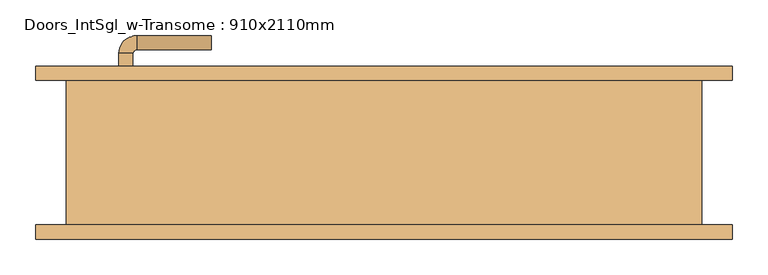
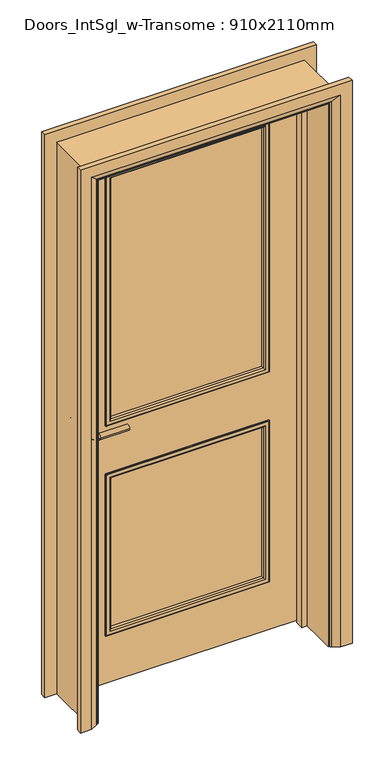
"""IFC4 building model written with IfcOpenShell, lengths in millimetres: door geometry, Doors_IntSgl_w-Transome : 910x2110mm."""

from ifc_helpers import new_model, si_unit, point, frame, frame_2d, origin, place, context, project, spatial, polyline, circle_curve, ellipse_curve, trimmed, segment, composite_curve, outline, extrude, faceted_brep, source, transform, mapped, element, save
from ifc_brep_helpers import plane_surface, cylinder_surface, revolved_surface, advanced_brep


def doors_intsgl_w_transome_910x2110mm_0d7ac49b(model_context):
    return source(origin(), model_context, "Body", "SolidModel", [
        advanced_brep(
        [(-373.0, 55.6, 1000.0), (-353.0, 55.6, 1000.0), (-353.0, 25.6, 1000.0), (-373.0, 25.6, 1000.0), (-348.0, 20.6, 1000.0), (-348.0, 0.6, 1000.0), (-243.0, 0.6, 1000.0), (-243.0, 20.6, 1000.0)],
        [
            (0, 1, circle_curve(frame((-363.0, 55.6, 1000.0), z_axis=(0.0, 1.0, 0.0), x_axis=(1.0, 0.0, 0.0)), 10.0)),
            (1, 0, circle_curve(frame((-363.0, 55.6, 1000.0), z_axis=(0.0, 1.0, 0.0), x_axis=(1.0, 0.0, 0.0)), 10.0)),
            (1, 2),
            (2, 3, circle_curve(frame((-363.0, 25.6, 1000.0), z_axis=(0.0, 1.0, 0.0), x_axis=(1.0, 0.0, 0.0)), 10.0)),
            (3, 0),
            (3, 2, circle_curve(frame((-363.0, 25.6, 1000.0), z_axis=(0.0, 1.0, 0.0), x_axis=(1.0, 0.0, 0.0)), 10.0)),
            (4, 5, circle_curve(frame((-348.0, 10.6, 1000.0), z_axis=(-1.0, 0.0, 0.0), x_axis=(0.0, 1.0, 0.0)), 10.0)),
            (5, 3, circle_curve(frame((-348.0, 25.6, 1000.0), z_axis=(0.0, 0.0, -1.0), x_axis=(-1.0, 0.0, 0.0)), 25.0)),
            (2, 4, circle_curve(frame((-348.0, 25.6, 1000.0), z_axis=(0.0, 0.0, 1.0), x_axis=(-1.0, 0.0, 0.0)), 5.0)),
            (5, 4, circle_curve(frame((-348.0, 10.6, 1000.0), z_axis=(-1.0, 0.0, 0.0), x_axis=(0.0, 1.0, 0.0)), 10.0)),
            (6, 7, circle_curve(frame((-243.0, 10.6, 1000.0), z_axis=(1.0, 0.0, 0.0), x_axis=(0.0, 1.0, 0.0)), 10.0)),
            (7, 6, circle_curve(frame((-243.0, 10.6, 1000.0), z_axis=(1.0, 0.0, 0.0), x_axis=(0.0, 1.0, 0.0)), 10.0)),
            (4, 7),
            (6, 5),
        ],
        [
            plane_surface(frame((-363.0, 55.6, 1000.0), z_axis=(0.0, 1.0, 0.0), x_axis=(0.0, 0.0, 1.0))),
            cylinder_surface(frame((-363.0, 55.6, 1000.0), z_axis=(0.0, 1.0, 0.0), x_axis=(1.0, 0.0, 0.0)), 10.0),
            revolved_surface(trimmed(ellipse_curve(frame((-363.0, 25.6, 1000.0), z_axis=(0.0, -1.0, 0.0), x_axis=(1.0, 0.0, 0.0)), 10.0, 10.0), [point((-373.0, 25.6, 1000.0))], [point((-353.0, 25.6, 1000.0))], True, "CARTESIAN"), (-348.0, 25.6, 1000.0), (0.0, 0.0, -1.0)),
            revolved_surface(trimmed(ellipse_curve(frame((-363.0, 25.6, 1000.0), z_axis=(0.0, -1.0, 0.0), x_axis=(1.0, 0.0, 0.0)), 10.0, 10.0), [point((-353.0, 25.6, 1000.0))], [point((-373.0, 25.6, 1000.0))], True, "CARTESIAN"), (-348.0, 25.6, 1000.0), (0.0, 0.0, -1.0)),
            plane_surface(frame((-243.0, 10.6, 1000.0), z_axis=(1.0, 0.0, 0.0), x_axis=(0.0, 0.0, 1.0))),
            cylinder_surface(frame((-348.0, 10.6, 1000.0), z_axis=(-1.0, 0.0, 0.0), x_axis=(0.0, 1.0, 0.0)), 10.0),
        ],
        [
            (0, [[1, 2]]),
            (1, [[3, 4, 5, -2]]),
            (1, [[-5, 6, -3, -1]]),
            (2, [[7, 8, -4, 9]]),
            (3, [[10, -9, -6, -8]]),
            (4, [[11, 12]]),
            (5, [[13, -11, 14, -7]]),
            (5, [[-14, -12, -13, -10]]),
        ],
    ),
        extrude(outline(composite_curve([segment(trimmed(circle_curve(frame_2d((1000.0, -365.5)), 30.0), [point((1000.0, -395.5))], [point((1000.0, -335.5))], False, "CARTESIAN"), True, "CONTINUOUS"), segment(trimmed(circle_curve(frame_2d((1000.0, -365.5)), 30.0), [point((1000.0, -335.5))], [point((1000.0, -395.5))], False, "CARTESIAN"), True, "CONTINUOUS")], self_intersect=False)), frame((0.0, 55.6, 0.0), z_axis=(0.0, 1.0, 0.0), x_axis=(0.0, 0.0, 1.0)), (0.0, 0.0, 1.0), 8.0),
        advanced_brep(
        [(-373.0, 109.6, 1000.0), (-353.0, 109.6, 1000.0), (-373.0, 139.6, 1000.0), (-353.0, 139.6, 1000.0), (-348.0, 144.6, 1000.0), (-348.0, 164.6, 1000.0), (-243.0, 164.6, 1000.0), (-243.0, 144.6, 1000.0)],
        [
            (0, 1, circle_curve(frame((-363.0, 109.6, 1000.0), z_axis=(0.0, -1.0, 0.0), x_axis=(1.0, 0.0, 0.0)), 10.0)),
            (1, 0, circle_curve(frame((-363.0, 109.6, 1000.0), z_axis=(0.0, -1.0, 0.0), x_axis=(1.0, 0.0, 0.0)), 10.0)),
            (0, 2),
            (2, 3, circle_curve(frame((-363.0, 139.6, 1000.0), z_axis=(0.0, -1.0, 0.0), x_axis=(1.0, 0.0, 0.0)), 10.0)),
            (3, 1),
            (3, 2, circle_curve(frame((-363.0, 139.6, 1000.0), z_axis=(0.0, -1.0, 0.0), x_axis=(1.0, 0.0, 0.0)), 10.0)),
            (4, 3, circle_curve(frame((-348.0, 139.6, 1000.0), z_axis=(0.0, 0.0, 1.0), x_axis=(-1.0, 0.0, 0.0)), 5.0)),
            (2, 5, circle_curve(frame((-348.0, 139.6, 1000.0), z_axis=(0.0, 0.0, -1.0), x_axis=(-1.0, 0.0, 0.0)), 25.0)),
            (5, 4, circle_curve(frame((-348.0, 154.6, 1000.0), z_axis=(-1.0, 0.0, 0.0), x_axis=(0.0, -1.0, 0.0)), 10.0)),
            (4, 5, circle_curve(frame((-348.0, 154.6, 1000.0), z_axis=(-1.0, 0.0, 0.0), x_axis=(0.0, -1.0, 0.0)), 10.0)),
            (6, 7, circle_curve(frame((-243.0, 154.6, 1000.0), z_axis=(1.0, 0.0, 0.0), x_axis=(0.0, -1.0, 0.0)), 10.0)),
            (7, 6, circle_curve(frame((-243.0, 154.6, 1000.0), z_axis=(1.0, 0.0, 0.0), x_axis=(0.0, -1.0, 0.0)), 10.0)),
            (5, 6),
            (7, 4),
        ],
        [
            plane_surface(frame((-363.0, 109.6, 1000.0), z_axis=(0.0, -1.0, 0.0), x_axis=(0.0, 0.0, 1.0))),
            cylinder_surface(frame((-363.0, 109.6, 1000.0), z_axis=(0.0, -1.0, 0.0), x_axis=(1.0, 0.0, 0.0)), 10.0),
            revolved_surface(trimmed(ellipse_curve(frame((-363.0, 139.6, 1000.0), z_axis=(0.0, -1.0, 0.0), x_axis=(1.0, 0.0, 0.0)), 10.0, 10.0), [point((-373.0, 139.6, 1000.0))], [point((-353.0, 139.6, 1000.0))], True, "CARTESIAN"), (-348.0, 139.6, 1000.0), (0.0, 0.0, -1.0)),
            revolved_surface(trimmed(ellipse_curve(frame((-363.0, 139.6, 1000.0), z_axis=(0.0, -1.0, 0.0), x_axis=(1.0, 0.0, 0.0)), 10.0, 10.0), [point((-353.0, 139.6, 1000.0))], [point((-373.0, 139.6, 1000.0))], True, "CARTESIAN"), (-348.0, 139.6, 1000.0), (0.0, 0.0, -1.0)),
            plane_surface(frame((-243.0, 154.6, 1000.0), z_axis=(1.0, 0.0, 0.0), x_axis=(0.0, 0.0, 1.0))),
            cylinder_surface(frame((-348.0, 154.6, 1000.0), z_axis=(-1.0, 0.0, 0.0), x_axis=(0.0, -1.0, 0.0)), 10.0),
        ],
        [
            (0, [[1, 2]]),
            (1, [[-1, 3, 4, 5]]),
            (1, [[-2, -5, 6, -3]]),
            (2, [[7, -4, 8, 9]]),
            (3, [[-8, -6, -7, 10]]),
            (4, [[11, 12]]),
            (5, [[-9, 13, -12, 14]]),
            (5, [[-10, -14, -11, -13]]),
        ],
    ),
        extrude(outline(composite_curve([segment(trimmed(circle_curve(frame_2d((1000.0, -365.5)), 30.0), [point((1000.0, -395.5))], [point((1000.0, -335.5))], False, "CARTESIAN"), True, "CONTINUOUS"), segment(trimmed(circle_curve(frame_2d((1000.0, -365.5)), 30.0), [point((1000.0, -335.5))], [point((1000.0, -395.5))], False, "CARTESIAN"), True, "CONTINUOUS")], self_intersect=False)), frame((0.0, 101.6, 0.0), z_axis=(0.0, 1.0, 0.0), x_axis=(0.0, 0.0, 1.0)), (0.0, 0.0, 1.0), 8.0),
        extrude(outline(polyline([(2068.0, -413.0), (8.0, -413.0), (8.0, 413.0), (2068.0, 413.0), (2068.0, -413.0)]), holes=[polyline([(1943.0, 288.0), (1000.0, 288.0), (1000.0, -288.0), (1943.0, -288.0), (1943.0, 288.0)]), polyline([(800.0, -288.0), (800.0, 288.0), (200.0, 288.0), (200.0, -288.0), (800.0, -288.0)])]), frame((0.0, 63.6, 0.0), z_axis=(0.0, 1.0, 0.0), x_axis=(0.0, 0.0, 1.0)), (0.0, 0.0, 1.0), 38.0),
        extrude(outline(polyline([(-288.0, 91.6), (288.0, 91.6), (288.0, 73.6), (-288.0, 73.6), (-288.0, 91.6)])), frame((0.0, 0.0, 1000.0), z_axis=(0.0, 0.0, 1.0), x_axis=(1.0, 0.0, 0.0)), (0.0, 0.0, 1.0), 943.0),
        extrude(outline(polyline([(-288.0, 91.6), (288.0, 91.6), (288.0, 73.6), (-288.0, 73.6), (-288.0, 91.6)])), frame((0.0, 0.0, 200.0), z_axis=(0.0, 0.0, 1.0), x_axis=(1.0, 0.0, 0.0)), (0.0, 0.0, 1.0), 600.0),
        faceted_brep([(-415.0, 101.6, 0.0), (-415.0, -101.6, 0.0), (-447.0, -101.6, 0.0), (-447.0, 101.6, 0.0), (-415.0, 101.6, 2070.0), (-415.0, -101.6, 2070.0), (-447.0, -101.6, 2102.0), (-447.0, 101.6, 2102.0), (415.0, 101.6, 0.0), (447.0, 101.6, 0.0), (447.0, -101.6, 0.0), (415.0, -101.6, 0.0), (415.0, 101.6, 2070.0), (447.0, 101.6, 2102.0), (447.0, -101.6, 2102.0), (415.0, -101.6, 2070.0)], [[[0, 1, 2, 3]], [[1, 0, 4, 5]], [[2, 1, 5, 6]], [[3, 2, 6, 7]], [[0, 3, 7, 4]], [[8, 9, 10, 11]], [[12, 13, 9, 8]], [[13, 14, 10, 9]], [[14, 15, 11, 10]], [[15, 12, 8, 11]], [[5, 4, 12, 15]], [[6, 5, 15, 14]], [[7, 6, 14, 13]], [[4, 7, 13, 12]]]),
        extrude(outline(polyline([(0.0, -415.0), (0.0, -396.0), (2051.0, -396.0), (2051.0, 396.0), (0.0, 396.0), (0.0, 415.0), (2070.0, 415.0), (2070.0, -415.0), (0.0, -415.0)])), frame((0.0, 29.6, 0.0), z_axis=(0.0, 1.0, 0.0), x_axis=(0.0, 0.0, 1.0)), (0.0, 0.0, 1.0), 32.0),
        advanced_brep(
        [(-490.0, -121.6, 0.0), (-490.0, -101.6, 0.0), (-420.0, -101.6, 0.0), (-424.0, -107.6, 0.0), (-450.0, -121.6, 0.0), (-490.0, -121.6, 2145.0), (-490.0, -101.6, 2145.0), (490.0, -101.6, 2145.0), (490.0, -101.6, 0.0), (420.0, -101.6, 0.0), (420.0, -101.6, 2075.0), (-420.0, -101.6, 2075.0), (-424.0, -107.6, 2079.0), (-450.0, -121.6, 2105.0), (450.0, -121.6, 2105.0), (450.0, -121.6, 0.0), (490.0, -121.6, 0.0), (490.0, -121.6, 2145.0), (424.0, -107.6, 0.0), (424.0, -107.6, 2079.0)],
        [
            (0, 1),
            (1, 2),
            (2, 3, circle_curve(frame((-428.0, -100.6, 0.0), z_axis=(0.0, 0.0, -1.0), x_axis=(-1.0, 0.0, 0.0)), 8.0622577)),
            (3, 4),
            (4, 0),
            (0, 5),
            (5, 6),
            (6, 1),
            (6, 7),
            (7, 8),
            (8, 9),
            (9, 10),
            (10, 11),
            (11, 2),
            (11, 12, ellipse_curve(frame((-428.0, -100.6, 2083.0), z_axis=(-0.7071067811865475, 0.0, -0.7071067811865475), x_axis=(0.7071067811865474, 0.0, -0.7071067811865476)), 11.4017543, 8.0622577)),
            (12, 3),
            (12, 13),
            (13, 4),
            (13, 14),
            (14, 15),
            (15, 16),
            (16, 17),
            (17, 5),
            (7, 17),
            (16, 8),
            (15, 18),
            (18, 9, circle_curve(frame((428.0, -100.6, 0.0), z_axis=(0.0, 0.0, -1.0), x_axis=(1.0, 0.0, 0.0)), 8.0622577)),
            (19, 10, ellipse_curve(frame((428.0, -100.6, 2083.0), z_axis=(0.7071067811865475, 0.0, -0.7071067811865475), x_axis=(0.7071067811865474, 0.0, 0.7071067811865476)), 11.4017543, 8.0622577)),
            (18, 19),
            (14, 19),
            (19, 12),
        ],
        [
            plane_surface(frame((-420.0, -101.6, 0.0), z_axis=(0.0, 0.0, -1.0), x_axis=(0.0, -1.0, 0.0))),
            plane_surface(frame((-490.0, -121.6, 0.0), z_axis=(-1.0, 0.0, 0.0), x_axis=(0.0, 0.0, 1.0))),
            plane_surface(frame((-490.0, -101.6, 0.0), z_axis=(0.0, 1.0, 0.0), x_axis=(0.0, 0.0, 1.0))),
            cylinder_surface(frame((-428.0, -100.6, 0.0), z_axis=(0.0, 0.0, -1.0), x_axis=(-1.0, 0.0, 0.0)), 8.0622577),
            plane_surface(frame((-424.0, -107.6, 0.0), z_axis=(0.4740998230350183, -0.8804710999221749, 0.0), x_axis=(0.0, 0.0, 1.0))),
            plane_surface(frame((-450.0, -121.6, 0.0), z_axis=(0.0, -1.0, 0.0), x_axis=(0.0, 0.0, 1.0))),
            plane_surface(frame((490.0, -121.6, 2145.0), z_axis=(1.0, 0.0, 0.0), x_axis=(0.0, 0.0, -1.0))),
            plane_surface(frame((420.0, -101.6, 0.0), z_axis=(0.0, 0.0, -1.0), x_axis=(0.0, -1.0, 0.0))),
            cylinder_surface(frame((428.0, -100.6, 2075.0), z_axis=(0.0, 0.0, 1.0), x_axis=(1.0, 0.0, 0.0)), 8.0622577),
            plane_surface(frame((424.0, -107.6, 2079.0), z_axis=(-0.4740998230350183, -0.8804710999221749, 0.0), x_axis=(0.0, 0.0, -1.0))),
            plane_surface(frame((-490.0, -121.6, 2145.0), z_axis=(0.0, 0.0, 1.0), x_axis=(1.0, 0.0, 0.0))),
            cylinder_surface(frame((-420.0, -100.6, 2083.0), z_axis=(-1.0, 0.0, 0.0), x_axis=(0.0, 0.0, 1.0)), 8.0622577),
            plane_surface(frame((-424.0, -107.6, 2079.0), z_axis=(0.0, -0.8804710999221749, -0.4740998230350183), x_axis=(1.0, 0.0, 0.0))),
        ],
        [
            (0, [[1, 2, 3, 4, 5]]),
            (1, [[-1, 6, 7, 8]]),
            (2, [[-2, -8, 9, 10, 11, 12, 13, 14]]),
            (3, [[-3, -14, 15, 16]]),
            (4, [[-4, -16, 17, 18]]),
            (5, [[-5, -18, 19, 20, 21, 22, 23, -6]]),
            (6, [[24, -22, 25, -10]]),
            (7, [[-21, 26, 27, -11, -25]]),
            (8, [[28, -12, -27, 29]]),
            (9, [[30, -29, -26, -20]]),
            (10, [[-7, -23, -24, -9]]),
            (11, [[-15, -13, -28, 31]]),
            (12, [[-17, -31, -30, -19]]),
        ],
    ),
        advanced_brep(
        [(490.0, 121.6, 0.0), (490.0, 101.6, 0.0), (420.0, 101.6, 0.0), (424.0, 107.6, 0.0), (450.0, 121.6, 0.0), (490.0, 121.6, 2145.0), (490.0, 101.6, 2145.0), (-490.0, 101.6, 2145.0), (-490.0, 101.6, 0.0), (-420.0, 101.6, 0.0), (-420.0, 101.6, 2075.0), (420.0, 101.6, 2075.0), (424.0, 107.6, 2079.0), (450.0, 121.6, 2105.0), (-450.0, 121.6, 2105.0), (-450.0, 121.6, 0.0), (-490.0, 121.6, 0.0), (-490.0, 121.6, 2145.0), (-424.0, 107.6, 0.0), (-424.0, 107.6, 2079.0)],
        [
            (0, 1),
            (1, 2),
            (2, 3, circle_curve(frame((428.0, 100.6, 0.0), z_axis=(0.0, 0.0, -1.0), x_axis=(1.0, 0.0, 0.0)), 8.0622577)),
            (3, 4),
            (4, 0),
            (0, 5),
            (5, 6),
            (6, 1),
            (6, 7),
            (7, 8),
            (8, 9),
            (9, 10),
            (10, 11),
            (11, 2),
            (11, 12, ellipse_curve(frame((428.0, 100.6, 2083.0), z_axis=(0.7071067811865475, 0.0, -0.7071067811865475), x_axis=(-0.7071067811865474, 0.0, -0.7071067811865476)), 11.4017543, 8.0622577)),
            (12, 3),
            (12, 13),
            (13, 4),
            (13, 14),
            (14, 15),
            (15, 16),
            (16, 17),
            (17, 5),
            (7, 17),
            (16, 8),
            (15, 18),
            (18, 9, circle_curve(frame((-428.0, 100.6, 0.0), z_axis=(0.0, 0.0, -1.0), x_axis=(-1.0, 0.0, 0.0)), 8.0622577)),
            (19, 10, ellipse_curve(frame((-428.0, 100.6, 2083.0), z_axis=(-0.7071067811865475, 0.0, -0.7071067811865475), x_axis=(-0.7071067811865474, 0.0, 0.7071067811865476)), 11.4017543, 8.0622577)),
            (18, 19),
            (14, 19),
            (19, 12),
        ],
        [
            plane_surface(frame((420.0, 101.6, 0.0), z_axis=(0.0, 0.0, -1.0), x_axis=(0.0, -1.0, 0.0))),
            plane_surface(frame((490.0, 121.6, 0.0), z_axis=(1.0, 0.0, 0.0), x_axis=(0.0, 0.0, 1.0))),
            plane_surface(frame((490.0, 101.6, 0.0), z_axis=(0.0, -1.0, 0.0), x_axis=(0.0, 0.0, 1.0))),
            cylinder_surface(frame((428.0, 100.6, 0.0), z_axis=(0.0, 0.0, -1.0), x_axis=(1.0, 0.0, 0.0)), 8.0622577),
            plane_surface(frame((424.0, 107.6, 0.0), z_axis=(-0.4740998230350126, 0.880471099922178, 0.0), x_axis=(0.0, 0.0, 1.0))),
            plane_surface(frame((450.0, 121.6, 0.0), z_axis=(0.0, 1.0, 0.0), x_axis=(0.0, 0.0, 1.0))),
            plane_surface(frame((-490.0, 121.6, 2145.0), z_axis=(-1.0, 0.0, 0.0), x_axis=(0.0, 0.0, -1.0))),
            plane_surface(frame((-420.0, 101.6, 0.0), z_axis=(0.0, 0.0, -1.0), x_axis=(0.0, -1.0, 0.0))),
            cylinder_surface(frame((-428.0, 100.6, 2075.0), z_axis=(0.0, 0.0, 1.0), x_axis=(-1.0, 0.0, 0.0)), 8.0622577),
            plane_surface(frame((-424.0, 107.6, 2079.0), z_axis=(0.47409982303501824, 0.8804710999221749, 0.0), x_axis=(0.0, 0.0, -1.0))),
            plane_surface(frame((490.0, 121.6, 2145.0), z_axis=(0.0, 0.0, 1.0), x_axis=(-1.0, 0.0, 0.0))),
            cylinder_surface(frame((420.0, 100.6, 2083.0), z_axis=(1.0, 0.0, 0.0), x_axis=(0.0, 0.0, 1.0)), 8.0622577),
            plane_surface(frame((424.0, 107.6, 2079.0), z_axis=(0.0, 0.8804710999221764, -0.4740998230350154), x_axis=(-1.0, 0.0, 0.0))),
        ],
        [
            (0, [[1, 2, 3, 4, 5]]),
            (1, [[-1, 6, 7, 8]]),
            (2, [[-2, -8, 9, 10, 11, 12, 13, 14]]),
            (3, [[-3, -14, 15, 16]]),
            (4, [[-4, -16, 17, 18]]),
            (5, [[-5, -18, 19, 20, 21, 22, 23, -6]]),
            (6, [[24, -22, 25, -10]]),
            (7, [[-21, 26, 27, -11, -25]]),
            (8, [[28, -12, -27, 29]]),
            (9, [[30, -29, -26, -20]]),
            (10, [[-7, -23, -24, -9]]),
            (11, [[-15, -13, -28, 31]]),
            (12, [[-17, -31, -30, -19]]),
        ],
    ),
        advanced_brep(
        [(-288.0, 91.6, 1943.0), (-288.0, 101.6, 1943.0), (-288.0, 101.6, 1000.0), (-288.0, 91.6, 1000.0), (-276.0, 102.6, 1931.0), (-276.0, 91.6, 1931.0), (-276.0, 91.6, 1012.0), (-276.0, 102.6, 1012.0), (-281.0, 107.6, 1936.0), (-281.0, 107.6, 1007.0), (-296.0, 105.6, 1951.0), (-294.0, 107.6, 1949.0), (-294.0, 107.6, 994.0), (-296.0, 105.6, 992.0), (-296.0, 101.6, 1951.0), (-296.0, 101.6, 992.0), (288.0, 101.6, 1000.0), (288.0, 91.6, 1000.0), (276.0, 91.6, 1012.0), (276.0, 102.6, 1012.0), (281.0, 107.6, 1007.0), (294.0, 107.6, 994.0), (296.0, 105.6, 992.0), (296.0, 101.6, 992.0), (288.0, 101.6, 1943.0), (288.0, 91.6, 1943.0), (276.0, 91.6, 1931.0), (276.0, 102.6, 1931.0), (281.0, 107.6, 1936.0), (294.0, 107.6, 1949.0), (296.0, 105.6, 1951.0), (296.0, 101.6, 1951.0)],
        [
            (0, 1),
            (1, 2),
            (2, 3),
            (3, 0),
            (4, 5),
            (5, 6),
            (6, 7),
            (7, 4),
            (8, 4, ellipse_curve(frame((-281.0, 102.6, 1936.0), z_axis=(-0.7071067811865475, 0.0, -0.7071067811865475), x_axis=(-0.7071067811865474, 0.0, 0.7071067811865476)), 7.0710678, 5.0)),
            (7, 9, ellipse_curve(frame((-281.0, 102.6, 1007.0), z_axis=(-0.7071067811865475, 0.0, 0.7071067811865475), x_axis=(0.7071067811865474, 0.0, 0.7071067811865476)), 7.0710678, 5.0)),
            (9, 8),
            (10, 11, ellipse_curve(frame((-294.0, 105.6, 1949.0), z_axis=(-0.7071067811865475, 0.0, -0.7071067811865475), x_axis=(-0.7071067811865474, 0.0, 0.7071067811865476)), 2.8284271, 2.0)),
            (11, 12),
            (12, 13, ellipse_curve(frame((-294.0, 105.6, 994.0), z_axis=(-0.7071067811865475, 0.0, 0.7071067811865475), x_axis=(0.7071067811865474, 0.0, 0.7071067811865476)), 2.8284271, 2.0)),
            (13, 10),
            (14, 10),
            (13, 15),
            (15, 14),
            (2, 16),
            (16, 17),
            (17, 3),
            (6, 18),
            (18, 19),
            (19, 7),
            (19, 20, ellipse_curve(frame((281.0, 102.6, 1007.0), z_axis=(-0.7071067811865475, 0.0, -0.7071067811865475), x_axis=(-0.7071067811865476, 0.0, 0.7071067811865474)), 7.0710678, 5.0)),
            (20, 9),
            (12, 21),
            (21, 22, ellipse_curve(frame((294.0, 105.6, 994.0), z_axis=(-0.7071067811865475, 0.0, -0.7071067811865475), x_axis=(-0.7071067811865476, 0.0, 0.7071067811865474)), 2.8284271, 2.0)),
            (22, 13),
            (22, 23),
            (23, 15),
            (16, 24),
            (24, 25),
            (25, 17),
            (18, 26),
            (26, 27),
            (27, 19),
            (27, 28, ellipse_curve(frame((281.0, 102.6, 1936.0), z_axis=(0.7071067811865475, 0.0, -0.7071067811865475), x_axis=(-0.7071067811865474, 0.0, -0.7071067811865476)), 7.0710678, 5.0)),
            (28, 20),
            (21, 29),
            (29, 30, ellipse_curve(frame((294.0, 105.6, 1949.0), z_axis=(0.7071067811865475, 0.0, -0.7071067811865475), x_axis=(-0.7071067811865474, 0.0, -0.7071067811865476)), 2.8284271, 2.0)),
            (30, 22),
            (30, 31),
            (31, 23),
            (31, 14),
            (1, 24),
            (0, 25),
            (5, 26),
            (4, 27),
            (8, 28),
            (11, 29),
            (10, 30),
        ],
        [
            plane_surface(frame((-288.0, 101.6, 1943.0), z_axis=(-1.0, 0.0, 0.0), x_axis=(0.0, 0.0, -1.0))),
            plane_surface(frame((-276.0, 91.6, 1931.0), z_axis=(1.0, 0.0, 0.0), x_axis=(0.0, 0.0, -1.0))),
            cylinder_surface(frame((-281.0, 102.6, 1943.0), z_axis=(0.0, 0.0, 1.0), x_axis=(-1.0, 0.0, 0.0)), 5.0),
            cylinder_surface(frame((-294.0, 105.6, 1943.0), z_axis=(0.0, 0.0, 1.0), x_axis=(-1.0, 0.0, 0.0)), 2.0),
            plane_surface(frame((-296.0, 105.6, 1951.0), z_axis=(-1.0, 0.0, 0.0), x_axis=(0.0, 0.0, -1.0))),
            plane_surface(frame((-288.0, 101.6, 1000.0), z_axis=(0.0, 0.0, -1.0), x_axis=(1.0, 0.0, 0.0))),
            plane_surface(frame((-276.0, 91.6, 1012.0), z_axis=(0.0, 0.0, 1.0), x_axis=(1.0, 0.0, 0.0))),
            cylinder_surface(frame((-288.0, 102.6, 1007.0), z_axis=(-1.0, 0.0, 0.0), x_axis=(0.0, 0.0, -1.0)), 5.0),
            cylinder_surface(frame((-288.0, 105.6, 994.0), z_axis=(-1.0, 0.0, 0.0), x_axis=(0.0, 0.0, -1.0)), 2.0),
            plane_surface(frame((-296.0, 105.6, 992.0), z_axis=(0.0, 0.0, -1.0), x_axis=(1.0, 0.0, 0.0))),
            plane_surface(frame((288.0, 101.6, 1000.0), z_axis=(1.0, 0.0, 0.0), x_axis=(0.0, 0.0, 1.0))),
            plane_surface(frame((276.0, 91.6, 1012.0), z_axis=(-1.0, 0.0, 0.0), x_axis=(0.0, 0.0, 1.0))),
            cylinder_surface(frame((281.0, 102.6, 1000.0), z_axis=(0.0, 0.0, -1.0), x_axis=(1.0, 0.0, 0.0)), 5.0),
            cylinder_surface(frame((294.0, 105.6, 1000.0), z_axis=(0.0, 0.0, -1.0), x_axis=(1.0, 0.0, 0.0)), 2.0),
            plane_surface(frame((296.0, 105.6, 992.0), z_axis=(1.0, 0.0, 0.0), x_axis=(0.0, 0.0, 1.0))),
            plane_surface(frame((296.0, 101.6, 1951.0), z_axis=(0.0, -1.0, 0.0), x_axis=(-1.0, 0.0, 0.0))),
            plane_surface(frame((288.0, 101.6, 1943.0), z_axis=(0.0, 0.0, 1.0), x_axis=(-1.0, 0.0, 0.0))),
            plane_surface(frame((288.0, 91.6, 1943.0), z_axis=(0.0, -1.0, 0.0), x_axis=(-1.0, 0.0, 0.0))),
            plane_surface(frame((276.0, 91.6, 1931.0), z_axis=(0.0, 0.0, -1.0), x_axis=(-1.0, 0.0, 0.0))),
            cylinder_surface(frame((288.0, 102.6, 1936.0), z_axis=(1.0, 0.0, 0.0), x_axis=(0.0, 0.0, 1.0)), 5.0),
            plane_surface(frame((281.0, 107.6, 1936.0), z_axis=(0.0, 1.0, 0.0), x_axis=(-1.0, 0.0, 0.0))),
            cylinder_surface(frame((288.0, 105.6, 1949.0), z_axis=(1.0, 0.0, 0.0), x_axis=(0.0, 0.0, 1.0)), 2.0),
            plane_surface(frame((296.0, 105.6, 1951.0), z_axis=(0.0, 0.0, 1.0), x_axis=(-1.0, 0.0, 0.0))),
        ],
        [
            (0, [[1, 2, 3, 4]]),
            (1, [[5, 6, 7, 8]]),
            (2, [[9, -8, 10, 11]]),
            (3, [[12, 13, 14, 15]]),
            (4, [[16, -15, 17, 18]]),
            (5, [[-3, 19, 20, 21]]),
            (6, [[-7, 22, 23, 24]]),
            (7, [[-10, -24, 25, 26]]),
            (8, [[-14, 27, 28, 29]]),
            (9, [[-17, -29, 30, 31]]),
            (10, [[-20, 32, 33, 34]]),
            (11, [[-23, 35, 36, 37]]),
            (12, [[-25, -37, 38, 39]]),
            (13, [[-28, 40, 41, 42]]),
            (14, [[-30, -42, 43, 44]]),
            (15, [[-31, -44, 45, -18], [46, -32, -19, -2]]),
            (16, [[-33, -46, -1, 47]]),
            (17, [[-21, -34, -47, -4], [48, -35, -22, -6]]),
            (18, [[-36, -48, -5, 49]]),
            (19, [[-38, -49, -9, 50]]),
            (20, [[51, -40, -27, -13], [-26, -39, -50, -11]]),
            (21, [[-41, -51, -12, 52]]),
            (22, [[-43, -52, -16, -45]]),
        ],
    ),
        advanced_brep(
        [(288.0, 73.6, 1943.0), (288.0, 63.6, 1943.0), (288.0, 63.6, 1000.0), (288.0, 73.6, 1000.0), (276.0, 62.6, 1931.0), (276.0, 73.6, 1931.0), (276.0, 73.6, 1012.0), (276.0, 62.6, 1012.0), (281.0, 57.6, 1936.0), (281.0, 57.6, 1007.0), (296.0, 59.6, 1951.0), (294.0, 57.6, 1949.0), (294.0, 57.6, 994.0), (296.0, 59.6, 992.0), (296.0, 63.6, 1951.0), (296.0, 63.6, 992.0), (-288.0, 63.6, 1000.0), (-288.0, 73.6, 1000.0), (-276.0, 73.6, 1012.0), (-276.0, 62.6, 1012.0), (-281.0, 57.6, 1007.0), (-294.0, 57.6, 994.0), (-296.0, 59.6, 992.0), (-296.0, 63.6, 992.0), (-288.0, 63.6, 1943.0), (-288.0, 73.6, 1943.0), (-276.0, 73.6, 1931.0), (-276.0, 62.6, 1931.0), (-281.0, 57.6, 1936.0), (-294.0, 57.6, 1949.0), (-296.0, 59.6, 1951.0), (-296.0, 63.6, 1951.0)],
        [
            (0, 1),
            (1, 2),
            (2, 3),
            (3, 0),
            (4, 5),
            (5, 6),
            (6, 7),
            (7, 4),
            (8, 4, ellipse_curve(frame((281.0, 62.6, 1936.0), z_axis=(0.7071067811865475, 0.0, -0.7071067811865475), x_axis=(0.7071067811865474, 0.0, 0.7071067811865476)), 7.0710678, 5.0)),
            (7, 9, ellipse_curve(frame((281.0, 62.6, 1007.0), z_axis=(0.7071067811865475, 0.0, 0.7071067811865475), x_axis=(-0.7071067811865474, 0.0, 0.7071067811865476)), 7.0710678, 5.0)),
            (9, 8),
            (10, 11, ellipse_curve(frame((294.0, 59.6, 1949.0), z_axis=(0.7071067811865475, 0.0, -0.7071067811865475), x_axis=(0.7071067811865474, 0.0, 0.7071067811865476)), 2.8284271, 2.0)),
            (11, 12),
            (12, 13, ellipse_curve(frame((294.0, 59.6, 994.0), z_axis=(0.7071067811865475, 0.0, 0.7071067811865475), x_axis=(-0.7071067811865474, 0.0, 0.7071067811865476)), 2.8284271, 2.0)),
            (13, 10),
            (14, 10),
            (13, 15),
            (15, 14),
            (2, 16),
            (16, 17),
            (17, 3),
            (6, 18),
            (18, 19),
            (19, 7),
            (19, 20, ellipse_curve(frame((-281.0, 62.6, 1007.0), z_axis=(0.7071067811865475, 0.0, -0.7071067811865475), x_axis=(0.7071067811865476, 0.0, 0.7071067811865474)), 7.0710678, 5.0)),
            (20, 9),
            (12, 21),
            (21, 22, ellipse_curve(frame((-294.0, 59.6, 994.0), z_axis=(0.7071067811865475, 0.0, -0.7071067811865475), x_axis=(0.7071067811865476, 0.0, 0.7071067811865474)), 2.8284271, 2.0)),
            (22, 13),
            (22, 23),
            (23, 15),
            (16, 24),
            (24, 25),
            (25, 17),
            (18, 26),
            (26, 27),
            (27, 19),
            (27, 28, ellipse_curve(frame((-281.0, 62.6, 1936.0), z_axis=(-0.7071067811865475, 0.0, -0.7071067811865475), x_axis=(0.7071067811865474, 0.0, -0.7071067811865476)), 7.0710678, 5.0)),
            (28, 20),
            (21, 29),
            (29, 30, ellipse_curve(frame((-294.0, 59.6, 1949.0), z_axis=(-0.7071067811865475, 0.0, -0.7071067811865475), x_axis=(0.7071067811865474, 0.0, -0.7071067811865476)), 2.8284271, 2.0)),
            (30, 22),
            (30, 31),
            (31, 23),
            (31, 14),
            (1, 24),
            (0, 25),
            (5, 26),
            (4, 27),
            (8, 28),
            (11, 29),
            (10, 30),
        ],
        [
            plane_surface(frame((288.0, 63.6, 1943.0), z_axis=(1.0, 0.0, 0.0), x_axis=(0.0, 0.0, -1.0))),
            plane_surface(frame((276.0, 73.6, 1931.0), z_axis=(-1.0, 0.0, 0.0), x_axis=(0.0, 0.0, -1.0))),
            cylinder_surface(frame((281.0, 62.6, 1943.0), z_axis=(0.0, 0.0, 1.0), x_axis=(1.0, 0.0, 0.0)), 5.0),
            cylinder_surface(frame((294.0, 59.6, 1943.0), z_axis=(0.0, 0.0, 1.0), x_axis=(1.0, 0.0, 0.0)), 2.0),
            plane_surface(frame((296.0, 59.6, 1951.0), z_axis=(1.0, 0.0, 0.0), x_axis=(0.0, 0.0, -1.0))),
            plane_surface(frame((288.0, 63.6, 1000.0), z_axis=(0.0, 0.0, -1.0), x_axis=(-1.0, 0.0, 0.0))),
            plane_surface(frame((276.0, 73.6, 1012.0), z_axis=(0.0, 0.0, 1.0), x_axis=(-1.0, 0.0, 0.0))),
            cylinder_surface(frame((288.0, 62.6, 1007.0), z_axis=(1.0, 0.0, 0.0), x_axis=(0.0, 0.0, -1.0)), 5.0),
            cylinder_surface(frame((288.0, 59.6, 994.0), z_axis=(1.0, 0.0, 0.0), x_axis=(0.0, 0.0, -1.0)), 2.0),
            plane_surface(frame((296.0, 59.6, 992.0), z_axis=(0.0, 0.0, -1.0), x_axis=(-1.0, 0.0, 0.0))),
            plane_surface(frame((-288.0, 63.6, 1000.0), z_axis=(-1.0, 0.0, 0.0), x_axis=(0.0, 0.0, 1.0))),
            plane_surface(frame((-276.0, 73.6, 1012.0), z_axis=(1.0, 0.0, 0.0), x_axis=(0.0, 0.0, 1.0))),
            cylinder_surface(frame((-281.0, 62.6, 1000.0), z_axis=(0.0, 0.0, -1.0), x_axis=(-1.0, 0.0, 0.0)), 5.0),
            cylinder_surface(frame((-294.0, 59.6, 1000.0), z_axis=(0.0, 0.0, -1.0), x_axis=(-1.0, 0.0, 0.0)), 2.0),
            plane_surface(frame((-296.0, 59.6, 992.0), z_axis=(-1.0, 0.0, 0.0), x_axis=(0.0, 0.0, 1.0))),
            plane_surface(frame((-296.0, 63.6, 1951.0), z_axis=(0.0, 1.0, 0.0), x_axis=(1.0, 0.0, 0.0))),
            plane_surface(frame((-288.0, 63.6, 1943.0), z_axis=(0.0, 0.0, 1.0), x_axis=(1.0, 0.0, 0.0))),
            plane_surface(frame((-288.0, 73.6, 1943.0), z_axis=(0.0, 1.0, 0.0), x_axis=(1.0, 0.0, 0.0))),
            plane_surface(frame((-276.0, 73.6, 1931.0), z_axis=(0.0, 0.0, -1.0), x_axis=(1.0, 0.0, 0.0))),
            cylinder_surface(frame((-288.0, 62.6, 1936.0), z_axis=(-1.0, 0.0, 0.0), x_axis=(0.0, 0.0, 1.0)), 5.0),
            plane_surface(frame((-281.0, 57.6, 1936.0), z_axis=(0.0, -1.0, 0.0), x_axis=(1.0, 0.0, 0.0))),
            cylinder_surface(frame((-288.0, 59.6, 1949.0), z_axis=(-1.0, 0.0, 0.0), x_axis=(0.0, 0.0, 1.0)), 2.0),
            plane_surface(frame((-296.0, 59.6, 1951.0), z_axis=(0.0, 0.0, 1.0), x_axis=(1.0, 0.0, 0.0))),
        ],
        [
            (0, [[1, 2, 3, 4]]),
            (1, [[5, 6, 7, 8]]),
            (2, [[9, -8, 10, 11]]),
            (3, [[12, 13, 14, 15]]),
            (4, [[16, -15, 17, 18]]),
            (5, [[-3, 19, 20, 21]]),
            (6, [[-7, 22, 23, 24]]),
            (7, [[-10, -24, 25, 26]]),
            (8, [[-14, 27, 28, 29]]),
            (9, [[-17, -29, 30, 31]]),
            (10, [[-20, 32, 33, 34]]),
            (11, [[-23, 35, 36, 37]]),
            (12, [[-25, -37, 38, 39]]),
            (13, [[-28, 40, 41, 42]]),
            (14, [[-30, -42, 43, 44]]),
            (15, [[-31, -44, 45, -18], [46, -32, -19, -2]]),
            (16, [[-33, -46, -1, 47]]),
            (17, [[-21, -34, -47, -4], [48, -35, -22, -6]]),
            (18, [[-36, -48, -5, 49]]),
            (19, [[-38, -49, -9, 50]]),
            (20, [[51, -40, -27, -13], [-26, -39, -50, -11]]),
            (21, [[-41, -51, -12, 52]]),
            (22, [[-43, -52, -16, -45]]),
        ],
    ),
        advanced_brep(
        [(296.0, 105.6, 808.0), (296.0, 101.6, 808.0), (296.0, 101.6, 192.0), (296.0, 105.6, 192.0), (294.0, 107.6, 806.0), (294.0, 107.6, 194.0), (276.0, 102.6, 788.0), (281.0, 107.6, 793.0), (281.0, 107.6, 207.0), (276.0, 102.6, 212.0), (276.0, 91.6, 788.0), (276.0, 91.6, 212.0), (288.0, 101.6, 800.0), (288.0, 91.6, 800.0), (288.0, 91.6, 200.0), (288.0, 101.6, 200.0), (-296.0, 101.6, 192.0), (-296.0, 105.6, 192.0), (-294.0, 107.6, 194.0), (-281.0, 107.6, 207.0), (-276.0, 102.6, 212.0), (-276.0, 91.6, 212.0), (-288.0, 91.6, 200.0), (-288.0, 101.6, 200.0), (-296.0, 101.6, 808.0), (-296.0, 105.6, 808.0), (-294.0, 107.6, 806.0), (-281.0, 107.6, 793.0), (-276.0, 102.6, 788.0), (-276.0, 91.6, 788.0), (-288.0, 91.6, 800.0), (-288.0, 101.6, 800.0)],
        [
            (0, 1),
            (1, 2),
            (2, 3),
            (3, 0),
            (4, 0, ellipse_curve(frame((294.0, 105.6, 806.0), z_axis=(0.7071067811865475, 0.0, -0.7071067811865475), x_axis=(0.7071067811865474, 0.0, 0.7071067811865476)), 2.8284271, 2.0)),
            (3, 5, ellipse_curve(frame((294.0, 105.6, 194.0), z_axis=(0.7071067811865475, 0.0, 0.7071067811865475), x_axis=(-0.7071067811865474, 0.0, 0.7071067811865476)), 2.8284271, 2.0)),
            (5, 4),
            (6, 7, ellipse_curve(frame((281.0, 102.6, 793.0), z_axis=(0.7071067811865475, 0.0, -0.7071067811865475), x_axis=(0.7071067811865474, 0.0, 0.7071067811865476)), 7.0710678, 5.0)),
            (7, 8),
            (8, 9, ellipse_curve(frame((281.0, 102.6, 207.0), z_axis=(0.7071067811865475, 0.0, 0.7071067811865475), x_axis=(-0.7071067811865474, 0.0, 0.7071067811865476)), 7.0710678, 5.0)),
            (9, 6),
            (10, 6),
            (9, 11),
            (11, 10),
            (12, 13),
            (13, 14),
            (14, 15),
            (15, 12),
            (2, 16),
            (16, 17),
            (17, 3),
            (17, 18, ellipse_curve(frame((-294.0, 105.6, 194.0), z_axis=(0.7071067811865475, 0.0, -0.7071067811865475), x_axis=(0.7071067811865476, 0.0, 0.7071067811865474)), 2.8284271, 2.0)),
            (18, 5),
            (8, 19),
            (19, 20, ellipse_curve(frame((-281.0, 102.6, 207.0), z_axis=(0.7071067811865475, 0.0, -0.7071067811865475), x_axis=(0.7071067811865476, 0.0, 0.7071067811865474)), 7.0710678, 5.0)),
            (20, 9),
            (20, 21),
            (21, 11),
            (14, 22),
            (22, 23),
            (23, 15),
            (16, 24),
            (24, 25),
            (25, 17),
            (25, 26, ellipse_curve(frame((-294.0, 105.6, 806.0), z_axis=(-0.7071067811865475, 0.0, -0.7071067811865475), x_axis=(0.7071067811865474, 0.0, -0.7071067811865476)), 2.8284271, 2.0)),
            (26, 18),
            (19, 27),
            (27, 28, ellipse_curve(frame((-281.0, 102.6, 793.0), z_axis=(-0.7071067811865475, 0.0, -0.7071067811865475), x_axis=(0.7071067811865474, 0.0, -0.7071067811865476)), 7.0710678, 5.0)),
            (28, 20),
            (28, 29),
            (29, 21),
            (22, 30),
            (30, 31),
            (31, 23),
            (24, 1),
            (0, 25),
            (4, 26),
            (7, 27),
            (6, 28),
            (10, 29),
            (13, 30),
            (12, 31),
        ],
        [
            plane_surface(frame((296.0, 101.6, 808.0), z_axis=(1.0, 0.0, 0.0), x_axis=(0.0, 0.0, -1.0))),
            cylinder_surface(frame((294.0, 105.6, 800.0), z_axis=(0.0, 0.0, 1.0), x_axis=(1.0, 0.0, 0.0)), 2.0),
            cylinder_surface(frame((281.0, 102.6, 800.0), z_axis=(0.0, 0.0, 1.0), x_axis=(1.0, 0.0, 0.0)), 5.0),
            plane_surface(frame((276.0, 102.6, 788.0), z_axis=(-1.0, 0.0, 0.0), x_axis=(0.0, 0.0, -1.0))),
            plane_surface(frame((288.0, 91.6, 800.0), z_axis=(1.0, 0.0, 0.0), x_axis=(0.0, 0.0, -1.0))),
            plane_surface(frame((296.0, 101.6, 192.0), z_axis=(0.0, 0.0, -1.0), x_axis=(-1.0, 0.0, 0.0))),
            cylinder_surface(frame((288.0, 105.6, 194.0), z_axis=(1.0, 0.0, 0.0), x_axis=(0.0, 0.0, -1.0)), 2.0),
            cylinder_surface(frame((288.0, 102.6, 207.0), z_axis=(1.0, 0.0, 0.0), x_axis=(0.0, 0.0, -1.0)), 5.0),
            plane_surface(frame((276.0, 102.6, 212.0), z_axis=(0.0, 0.0, 1.0), x_axis=(-1.0, 0.0, 0.0))),
            plane_surface(frame((288.0, 91.6, 200.0), z_axis=(0.0, 0.0, -1.0), x_axis=(-1.0, 0.0, 0.0))),
            plane_surface(frame((-296.0, 101.6, 192.0), z_axis=(-1.0, 0.0, 0.0), x_axis=(0.0, 0.0, 1.0))),
            cylinder_surface(frame((-294.0, 105.6, 200.0), z_axis=(0.0, 0.0, -1.0), x_axis=(-1.0, 0.0, 0.0)), 2.0),
            cylinder_surface(frame((-281.0, 102.6, 200.0), z_axis=(0.0, 0.0, -1.0), x_axis=(-1.0, 0.0, 0.0)), 5.0),
            plane_surface(frame((-276.0, 102.6, 212.0), z_axis=(1.0, 0.0, 0.0), x_axis=(0.0, 0.0, 1.0))),
            plane_surface(frame((-288.0, 91.6, 200.0), z_axis=(-1.0, 0.0, 0.0), x_axis=(0.0, 0.0, 1.0))),
            plane_surface(frame((-296.0, 101.6, 808.0), z_axis=(0.0, 0.0, 1.0), x_axis=(1.0, 0.0, 0.0))),
            cylinder_surface(frame((-288.0, 105.6, 806.0), z_axis=(-1.0, 0.0, 0.0), x_axis=(0.0, 0.0, 1.0)), 2.0),
            plane_surface(frame((-294.0, 107.6, 806.0), z_axis=(0.0, 1.0, 0.0), x_axis=(1.0, 0.0, 0.0))),
            cylinder_surface(frame((-288.0, 102.6, 793.0), z_axis=(-1.0, 0.0, 0.0), x_axis=(0.0, 0.0, 1.0)), 5.0),
            plane_surface(frame((-276.0, 102.6, 788.0), z_axis=(0.0, 0.0, -1.0), x_axis=(1.0, 0.0, 0.0))),
            plane_surface(frame((-276.0, 91.6, 788.0), z_axis=(0.0, -1.0, 0.0), x_axis=(1.0, 0.0, 0.0))),
            plane_surface(frame((-288.0, 91.6, 800.0), z_axis=(0.0, 0.0, 1.0), x_axis=(1.0, 0.0, 0.0))),
            plane_surface(frame((-288.0, 101.6, 800.0), z_axis=(0.0, -1.0, 0.0), x_axis=(1.0, 0.0, 0.0))),
        ],
        [
            (0, [[1, 2, 3, 4]]),
            (1, [[5, -4, 6, 7]]),
            (2, [[8, 9, 10, 11]]),
            (3, [[12, -11, 13, 14]]),
            (4, [[15, 16, 17, 18]]),
            (5, [[-3, 19, 20, 21]]),
            (6, [[-6, -21, 22, 23]]),
            (7, [[-10, 24, 25, 26]]),
            (8, [[-13, -26, 27, 28]]),
            (9, [[-17, 29, 30, 31]]),
            (10, [[-20, 32, 33, 34]]),
            (11, [[-22, -34, 35, 36]]),
            (12, [[-25, 37, 38, 39]]),
            (13, [[-27, -39, 40, 41]]),
            (14, [[-30, 42, 43, 44]]),
            (15, [[-33, 45, -1, 46]]),
            (16, [[-35, -46, -5, 47]]),
            (17, [[-23, -36, -47, -7], [48, -37, -24, -9]]),
            (18, [[-38, -48, -8, 49]]),
            (19, [[-40, -49, -12, 50]]),
            (20, [[51, -42, -29, -16], [-28, -41, -50, -14]]),
            (21, [[-43, -51, -15, 52]]),
            (22, [[-45, -32, -19, -2], [-31, -44, -52, -18]]),
        ],
    ),
        advanced_brep(
        [(288.0, 73.6, 800.0), (288.0, 63.6, 800.0), (288.0, 63.6, 200.0), (288.0, 73.6, 200.0), (276.0, 62.6, 788.0), (276.0, 73.6, 788.0), (276.0, 73.6, 212.0), (276.0, 62.6, 212.0), (281.0, 57.6, 793.0), (281.0, 57.6, 207.0), (296.0, 59.6, 808.0), (294.0, 57.6, 806.0), (294.0, 57.6, 194.0), (296.0, 59.6, 192.0), (296.0, 63.6, 808.0), (296.0, 63.6, 192.0), (-288.0, 63.6, 200.0), (-288.0, 73.6, 200.0), (-276.0, 73.6, 212.0), (-276.0, 62.6, 212.0), (-281.0, 57.6, 207.0), (-294.0, 57.6, 194.0), (-296.0, 59.6, 192.0), (-296.0, 63.6, 192.0), (-288.0, 63.6, 800.0), (-288.0, 73.6, 800.0), (-276.0, 73.6, 788.0), (-276.0, 62.6, 788.0), (-281.0, 57.6, 793.0), (-294.0, 57.6, 806.0), (-296.0, 59.6, 808.0), (-296.0, 63.6, 808.0)],
        [
            (0, 1),
            (1, 2),
            (2, 3),
            (3, 0),
            (4, 5),
            (5, 6),
            (6, 7),
            (7, 4),
            (8, 4, ellipse_curve(frame((281.0, 62.6, 793.0), z_axis=(0.7071067811865475, 0.0, -0.7071067811865475), x_axis=(0.7071067811865474, 0.0, 0.7071067811865476)), 7.0710678, 5.0)),
            (7, 9, ellipse_curve(frame((281.0, 62.6, 207.0), z_axis=(0.7071067811865475, 0.0, 0.7071067811865475), x_axis=(-0.7071067811865474, 0.0, 0.7071067811865476)), 7.0710678, 5.0)),
            (9, 8),
            (10, 11, ellipse_curve(frame((294.0, 59.6, 806.0), z_axis=(0.7071067811865475, 0.0, -0.7071067811865475), x_axis=(0.7071067811865474, 0.0, 0.7071067811865476)), 2.8284271, 2.0)),
            (11, 12),
            (12, 13, ellipse_curve(frame((294.0, 59.6, 194.0), z_axis=(0.7071067811865475, 0.0, 0.7071067811865475), x_axis=(-0.7071067811865474, 0.0, 0.7071067811865476)), 2.8284271, 2.0)),
            (13, 10),
            (14, 10),
            (13, 15),
            (15, 14),
            (2, 16),
            (16, 17),
            (17, 3),
            (6, 18),
            (18, 19),
            (19, 7),
            (19, 20, ellipse_curve(frame((-281.0, 62.6, 207.0), z_axis=(0.7071067811865475, 0.0, -0.7071067811865475), x_axis=(0.7071067811865476, 0.0, 0.7071067811865474)), 7.0710678, 5.0)),
            (20, 9),
            (12, 21),
            (21, 22, ellipse_curve(frame((-294.0, 59.6, 194.0), z_axis=(0.7071067811865475, 0.0, -0.7071067811865475), x_axis=(0.7071067811865476, 0.0, 0.7071067811865474)), 2.8284271, 2.0)),
            (22, 13),
            (22, 23),
            (23, 15),
            (16, 24),
            (24, 25),
            (25, 17),
            (18, 26),
            (26, 27),
            (27, 19),
            (27, 28, ellipse_curve(frame((-281.0, 62.6, 793.0), z_axis=(-0.7071067811865475, 0.0, -0.7071067811865475), x_axis=(0.7071067811865474, 0.0, -0.7071067811865476)), 7.0710678, 5.0)),
            (28, 20),
            (21, 29),
            (29, 30, ellipse_curve(frame((-294.0, 59.6, 806.0), z_axis=(-0.7071067811865475, 0.0, -0.7071067811865475), x_axis=(0.7071067811865474, 0.0, -0.7071067811865476)), 2.8284271, 2.0)),
            (30, 22),
            (30, 31),
            (31, 23),
            (31, 14),
            (1, 24),
            (0, 25),
            (5, 26),
            (4, 27),
            (8, 28),
            (11, 29),
            (10, 30),
        ],
        [
            plane_surface(frame((288.0, 63.6, 800.0), z_axis=(1.0, 0.0, 0.0), x_axis=(0.0, 0.0, -1.0))),
            plane_surface(frame((276.0, 73.6, 788.0), z_axis=(-1.0, 0.0, 0.0), x_axis=(0.0, 0.0, -1.0))),
            cylinder_surface(frame((281.0, 62.6, 800.0), z_axis=(0.0, 0.0, 1.0), x_axis=(1.0, 0.0, 0.0)), 5.0),
            cylinder_surface(frame((294.0, 59.6, 800.0), z_axis=(0.0, 0.0, 1.0), x_axis=(1.0, 0.0, 0.0)), 2.0),
            plane_surface(frame((296.0, 59.6, 808.0), z_axis=(1.0, 0.0, 0.0), x_axis=(0.0, 0.0, -1.0))),
            plane_surface(frame((288.0, 63.6, 200.0), z_axis=(0.0, 0.0, -1.0), x_axis=(-1.0, 0.0, 0.0))),
            plane_surface(frame((276.0, 73.6, 212.0), z_axis=(0.0, 0.0, 1.0), x_axis=(-1.0, 0.0, 0.0))),
            cylinder_surface(frame((288.0, 62.6, 207.0), z_axis=(1.0, 0.0, 0.0), x_axis=(0.0, 0.0, -1.0)), 5.0),
            cylinder_surface(frame((288.0, 59.6, 194.0), z_axis=(1.0, 0.0, 0.0), x_axis=(0.0, 0.0, -1.0)), 2.0),
            plane_surface(frame((296.0, 59.6, 192.0), z_axis=(0.0, 0.0, -1.0), x_axis=(-1.0, 0.0, 0.0))),
            plane_surface(frame((-288.0, 63.6, 200.0), z_axis=(-1.0, 0.0, 0.0), x_axis=(0.0, 0.0, 1.0))),
            plane_surface(frame((-276.0, 73.6, 212.0), z_axis=(1.0, 0.0, 0.0), x_axis=(0.0, 0.0, 1.0))),
            cylinder_surface(frame((-281.0, 62.6, 200.0), z_axis=(0.0, 0.0, -1.0), x_axis=(-1.0, 0.0, 0.0)), 5.0),
            cylinder_surface(frame((-294.0, 59.6, 200.0), z_axis=(0.0, 0.0, -1.0), x_axis=(-1.0, 0.0, 0.0)), 2.0),
            plane_surface(frame((-296.0, 59.6, 192.0), z_axis=(-1.0, 0.0, 0.0), x_axis=(0.0, 0.0, 1.0))),
            plane_surface(frame((-296.0, 63.6, 808.0), z_axis=(0.0, 1.0, 0.0), x_axis=(1.0, 0.0, 0.0))),
            plane_surface(frame((-288.0, 63.6, 800.0), z_axis=(0.0, 0.0, 1.0), x_axis=(1.0, 0.0, 0.0))),
            plane_surface(frame((-288.0, 73.6, 800.0), z_axis=(0.0, 1.0, 0.0), x_axis=(1.0, 0.0, 0.0))),
            plane_surface(frame((-276.0, 73.6, 788.0), z_axis=(0.0, 0.0, -1.0), x_axis=(1.0, 0.0, 0.0))),
            cylinder_surface(frame((-288.0, 62.6, 793.0), z_axis=(-1.0, 0.0, 0.0), x_axis=(0.0, 0.0, 1.0)), 5.0),
            plane_surface(frame((-281.0, 57.6, 793.0), z_axis=(0.0, -1.0, 0.0), x_axis=(1.0, 0.0, 0.0))),
            cylinder_surface(frame((-288.0, 59.6, 806.0), z_axis=(-1.0, 0.0, 0.0), x_axis=(0.0, 0.0, 1.0)), 2.0),
            plane_surface(frame((-296.0, 59.6, 808.0), z_axis=(0.0, 0.0, 1.0), x_axis=(1.0, 0.0, 0.0))),
        ],
        [
            (0, [[1, 2, 3, 4]]),
            (1, [[5, 6, 7, 8]]),
            (2, [[9, -8, 10, 11]]),
            (3, [[12, 13, 14, 15]]),
            (4, [[16, -15, 17, 18]]),
            (5, [[-3, 19, 20, 21]]),
            (6, [[-7, 22, 23, 24]]),
            (7, [[-10, -24, 25, 26]]),
            (8, [[-14, 27, 28, 29]]),
            (9, [[-17, -29, 30, 31]]),
            (10, [[-20, 32, 33, 34]]),
            (11, [[-23, 35, 36, 37]]),
            (12, [[-25, -37, 38, 39]]),
            (13, [[-28, 40, 41, 42]]),
            (14, [[-30, -42, 43, 44]]),
            (15, [[-31, -44, 45, -18], [46, -32, -19, -2]]),
            (16, [[-33, -46, -1, 47]]),
            (17, [[-21, -34, -47, -4], [48, -35, -22, -6]]),
            (18, [[-36, -48, -5, 49]]),
            (19, [[-38, -49, -9, 50]]),
            (20, [[51, -40, -27, -13], [-26, -39, -50, -11]]),
            (21, [[-41, -51, -12, 52]]),
            (22, [[-43, -52, -16, -45]]),
        ],
    ),
    ])


if __name__ == "__main__":
    model = new_model("IFC4")
    model_context = context("Model", 3, world=origin())
    ifc_project = project(units=[si_unit("LENGTHUNIT", "METRE", prefix="MILLI")], contexts=[model_context])
    site = spatial("IfcSite", under=ifc_project)
    building = spatial("IfcBuilding", under=site)
    placement = place(None, origin())
    doors_intsgl_w_transome_910x2110mm_shape = doors_intsgl_w_transome_910x2110mm_0d7ac49b(model_context)
    element("IfcDoor", 1, ObjectType="Doors_IntSgl_w-Transome : 910x2110mm", at=placement, inside=building, context=model_context, shape_type="MappedRepresentation", body=[
        mapped(doors_intsgl_w_transome_910x2110mm_shape, transform((0.0, 0.0, 0.0), x_axis=(1.0, 0.0, 0.0), y_axis=(0.0, 1.0, 0.0), z_axis=(0.0, 0.0, 1.0))),
    ])
    save(model, "model.ifc")

# Revit data of these elements
# Type "Doors_IntSgl_w-Transome : 910x2110mm"
#   Type Mark = "11"
#   Type Comments = "Internal Single"
#   Construction Type Id = "SGL"
#   Manufacturer = "Revit"
#   Keynote = "L20"
#   Description = "Internal Single Door"
#   Analytic Construction = "Large single-glazed windows"
#   Visual Light Transmittance = 0.9
#   UnderCut = 0' - 0.31496"
#   Top of Lock Rail = 3' - 3.37008"
#   Tolerance = 0' - 0.07874"
#   Thickness = 0' - 1.49606"
#   Structural Tolerance = 0' - 0.31496"
#   StopDepth = 0' - 1.25984"
#   Stop Thickness = 0' - 0.74803"
#   Stile Top Rail = 0' - 4.92126"
#   Stile Shutting = 0' - 4.92126"
#   Stile Lock Rail = 0' - 7.87402"
#   Stile Hanging = 0' - 4.92126"
#   Stile Bottom Rail = 0' - 7.87402"
#   Solar Heat Gain Coefficient = 0.86
#   Rough Width = 2' - 11.82677"
#   Rough Height = 6' - 11.07087"
#   Height to Top Lock Rail = 3' - 3.37008"
#   Heat Transfer Coefficient (U) = 0.979472 BTU/(h·ft²·°F)
#   Handle Z Distance = 3' - 3.37008"
#   Handle X Distance = 0' - 1.9685"
#   Frame Thickness = 0' - 1.25984"
#   Door Panel Width = 2' - 8.51969"
#   Door Panel Thickness = 0' - 1.49606"
#   Door Panel Offset = 0' - 0"
#   Height = 6' - 11.07087"
#   Width = 2' - 11.82677"
#   Door Panel Height = 6' - 9.10236"
#   Architrave Setback = 0' - 0.19685"
#   Vis - Ironmongery = yes
#   Define Thermal Properties by = 1
#   Material Ironmongery = Door - Handle
#   Material Glass = Door - Glazing
#   Material Frame = Door - Frame/Mullion
#   Material Door = Door - Panel
#   Material Beading = Door - Panel
#   Material Architrave = Door - Architrave
#   Function = (empty or 0)
#   Wall Closure = (empty or 0)
# Element 1 (IfcDoor, "Doors_IntSgl_w-Transome : 910x2110mm")
#   Materials on its faces: "Door - Panel", "Door - Architrave", "Door - Handle", "Door - Frame/Mullion", "Door - Glazing"
# Materials
#   "Door - Handle": colour RGB 247 247 247, transparency 0
#   "Door - Glazing": colour RGB 0 0 255, transparency 0.75
#   "Door - Frame/Mullion": class "Wood", colour RGB 212 179 113, transparency 0
#   "Door - Panel": class "Wood", colour RGB 210 159 95, transparency 0, Cost = 0
#   "Door - Architrave": class "Wood", colour RGB 154 90 5, transparency 0
